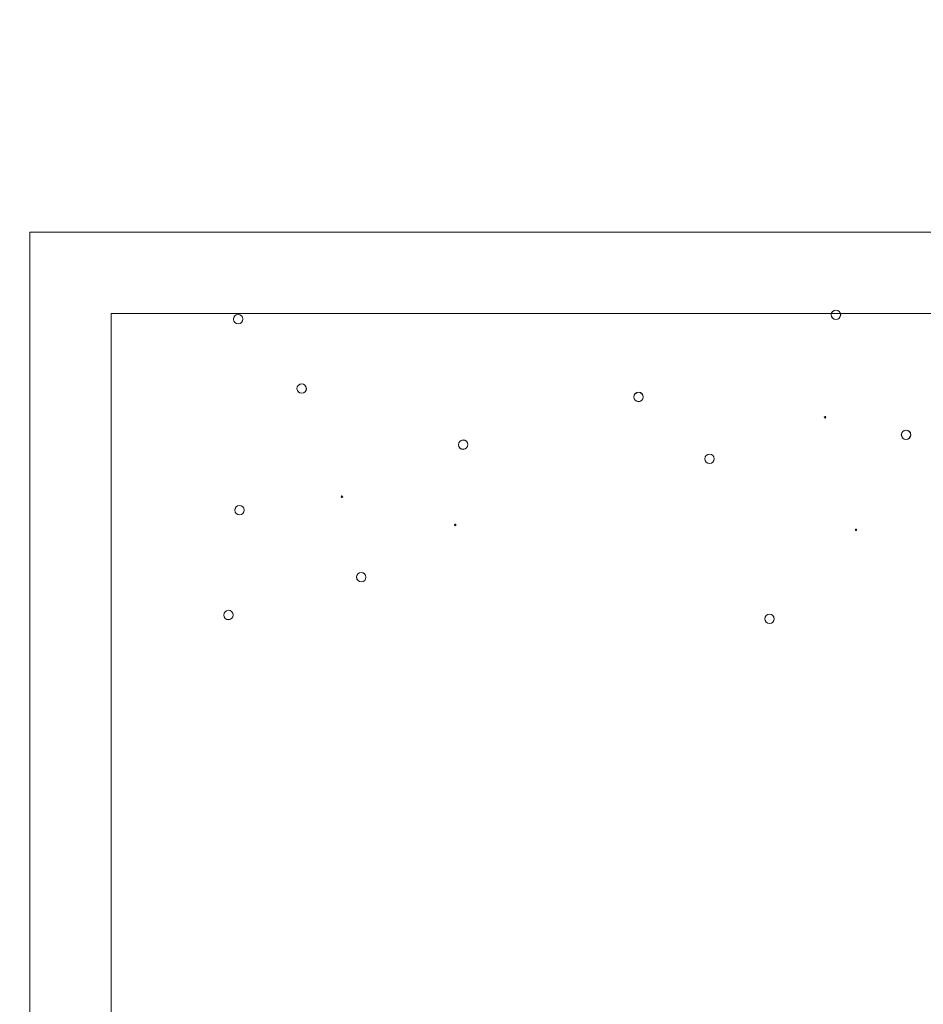
# Model space of a CAD drawing. Units: inches. Extents: x -466983 to 1020, y 324 to 318697.
# Tile 52 of 97: x 620.61 to 631.8, y 936.44 to 948.64. Entities that reach past the tile are written whole.
import ezdxf

# ---------------------------------------------------------------- set-up
doc = ezdxf.new("R2010")
doc.units = ezdxf.units.IN
doc.header["$MEASUREMENT"] = 0
doc.layers.add('A-FLOR-PATT', color=252, linetype='Continuous', lineweight=13)
doc.layers.add('A-FURN', color=8, linetype='Continuous', lineweight=18)

# ---------------------------------------------------------------- blocks, each defined once
blk = doc.blocks.new('L Shaped Sofa')
at = {"ltscale": 2}
for p, q in [((2458.96, 739.532), (2458.96, 802.773)), ((2460.8, 737.692), (2460.8, 802.773)), ((2458.96, 739.532), (2437.956, 739.532)), ((2460.8, 737.692), (2437.499, 737.692))]:
    blk.add_line(p, q, dxfattribs=at)
for centre, radius, start, end in [((2444.081, 746.436), 0.106, 90, 270), ((2444.081, 746.436), 0.106, 270, 90), ((2456.312, 746.349), 0.106, 1.3946, 181.3946), ((2456.312, 746.349), 0.106, 181.3946, 1.3946), ((2453.309, 745.494), 0.106, 1.3946, 181.3946), ((2453.309, 745.494), 0.106, 181.3946, 1.3946), ((2442.129, 744.423), 0.0177, 90, 270), ((2442.129, 744.423), 0.0177, 270, 90), ((2451.187, 744.312), 0.0177, 1.3946, 181.3946), ((2451.187, 744.312), 0.0177, 181.3946, 1.3946), ((2456.062, 743.978), 0.106, 1.3946, 181.3946), ((2456.062, 743.978), 0.106, 181.3946, 1.3946), ((2453.747, 743.675), 0.0177, 1.3946, 181.3946), ((2453.747, 743.675), 0.0177, 181.3946, 1.3946), ((2445.438, 742.815), 0.106, 90, 270), ((2445.438, 742.815), 0.106, 270, 90), ((2451.005, 742.498), 0.106, 1.3946, 181.3946), ((2451.005, 742.498), 0.106, 181.3946, 1.3946), ((2440.998, 742.273), 0.106, 90, 270), ((2440.998, 742.273), 0.106, 270, 90), ((2442.827, 741.879), 0.0177, 90, 270), ((2442.827, 741.879), 0.0177, 270, 90), ((2447.044, 741.419), 0.106, 90, 270), ((2447.044, 741.419), 0.106, 270, 90), ((2454.657, 741.23), 0.106, 1.3946, 181.3946), ((2454.657, 741.23), 0.106, 181.3946, 1.3946), ((2456.093, 739.658), 0.106, 1.3946, 181.3946), ((2442.581, 739.558), 0.106, 90, 270), ((2442.581, 739.558), 0.106, 270, 90), ((2456.093, 739.658), 0.106, 181.3946, 1.3946)]:
    blk.add_arc(centre, radius, start, end, dxfattribs=at)

msp = doc.modelspace()

# ---------------------------------------------------------------- hatches: boundary and pattern name
at = {"layer": 'A-FLOR-PATT', "transparency": 33554572}
h = msp.add_hatch(dxfattribs=at)
h.set_pattern_fill('ANSI37', color=256, scale=30)
h.set_pattern_definition([(45, (-1212.4137, -290.035), (-2.6516504, 2.6516504), []), (135, (-1212.4137, -290.035), (-2.6516504, -2.6516504), [])])
h.paths.add_polyline_path([(901.806, 1075.938), (900.614, 1075.938), (900.614, 1065.386), (899.391, 1065.386), (898.091, 1065.386), (892.836, 1058.71, -0.258377), (892.188, 1058.351), (879.985, 1058.351, -0.20177), (879.438, 1058.581), (874.081, 1065.386), (872.781, 1065.386), (871.558, 1065.386), (871.558, 1075.938), (813.806, 1075.938), (813.806, 1044.792), (832.395, 1044.792, -0.394795), (848.66, 1028.536), (848.66, 1009.938), (901.806, 1009.938), (901.806, 1015.938), (901.306, 1015.938), (871.306, 1015.938), (871.306, 1017.25), (871.334, 1017.25, -0.401453), (901.306, 1045.938), (901.806, 1045.938)])
edge = h.paths.add_edge_path(flags=16)
edge.add_line((847.773, 1068.949), (847.773, 1073.709))
edge.add_arc((849.227, 1073.709), 1.454, 90, 180, ccw=False)
edge.add_line((849.227, 1075.163), (864.492, 1075.163))
edge.add_arc((864.492, 1073.709), 1.454, 0, 90, ccw=False)
edge.add_line((865.946, 1073.709), (865.946, 1069.004))
edge.add_arc((832.645, 1068.976), 33.301, -20.6123, 0.0472, ccw=False)
edge.add_ellipse((856.859, 1058.48), major_axis=(0, 10.213), ratio=0.685919, start_angle=100.0088, end_angle=259.9912, ccw=False)
edge.add_arc((881.074, 1068.976), 33.301, 180.0472, 200.6123, ccw=False)
h.paths.add_polyline_path([(853.146, 1066.482), (853.146, 1066.453), (853.146, 1066.453, 0.433107), (852.917, 1066.685), (852.917, 1066.453), (853.146, 1066.453), (853.146, 1066.482), (853.088, 1066.612, 0.697939), (852.7, 1066.453), (852.7, 1066.453), (852.7, 1066.482), (852.917, 1067.001), (852.917, 1066.685, -0.396254)], flags=0)
h.paths.add_polyline_path([(861.019, 1066.482), (861.019, 1066.453), (861.019, 1066.453, 0.416404), (860.802, 1066.685), (860.802, 1066.453), (861.019, 1066.453), (861.019, 1066.482), (860.967, 1066.605, 0.713344), (860.573, 1066.453), (860.573, 1066.453), (860.573, 1066.482), (860.802, 1067.001), (860.802, 1066.685, -0.379973)], flags=0)
edge = h.paths.add_edge_path(flags=0)
edge.add_spline(control_points=[(861.13, 1065.785), (861.466, 1065.248), (861.613, 1065.016), (861.983, 1064.374), (862.192, 1063.944), (862.561, 1063.039), (862.721, 1062.563), (862.987, 1061.578), (863.092, 1061.069), (863.245, 1060.031), (863.293, 1059.503), (863.329, 1058.441), (863.318, 1057.908), (863.237, 1056.852), (863.166, 1056.329), (862.97, 1055.308), (862.843, 1054.81), (862.537, 1053.852), (862.357, 1053.393), (861.951, 1052.525), (861.725, 1052.117), (861.233, 1051.362), (860.967, 1051.016), (860.405, 1050.395), (860.108, 1050.12), (859.494, 1049.646), (859.176, 1049.448), (858.528, 1049.13), (858.197, 1049.011), (857.531, 1048.852), (857.196, 1048.812), (856.525, 1048.812), (856.189, 1048.852), (855.524, 1049.01), (855.193, 1049.129), (854.545, 1049.447), (854.227, 1049.645), (853.612, 1050.118), (853.316, 1050.393), (852.753, 1051.014), (852.487, 1051.36), (851.995, 1052.114), (851.769, 1052.523), (851.363, 1053.39), (851.183, 1053.85), (850.877, 1054.807), (850.75, 1055.305), (850.553, 1056.326), (850.483, 1056.849), (850.401, 1057.905), (850.39, 1058.438), (850.426, 1059.5), (850.473, 1060.028), (850.626, 1061.066), (850.732, 1061.575), (850.997, 1062.561), (851.157, 1063.036), (851.525, 1063.942), (851.734, 1064.371), (852.106, 1065.016), (852.254, 1065.25), (852.608, 1065.733)], knot_values=[3.915332, 3.915332, 3.915332, 3.915332, 4.013468, 4.013468, 4.175532, 4.175532, 4.337596, 4.337596, 4.49966, 4.49966, 4.661724, 4.661724, 4.823788, 4.823788, 4.985852, 4.985852, 5.147916, 5.147916, 5.30998, 5.30998, 5.472044, 5.472044, 5.634109, 5.634109, 5.796173, 5.796173, 5.958237, 5.958237, 6.120301, 6.120301, 6.282365, 6.282365, 6.444429, 6.444429, 6.606493, 6.606493, 6.768557, 6.768557, 6.930621, 6.930621, 7.092685, 7.092685, 7.254749, 7.254749, 7.416813, 7.416813, 7.578878, 7.578878, 7.740942, 7.740942, 7.903006, 7.903006, 8.06507, 8.06507, 8.227134, 8.227134, 8.389198, 8.389198, 8.551262, 8.551262, 8.65037, 8.65037, 8.65037, 8.65037], degree=3, periodic=0)
edge.add_line((852.642, 1065.785), (861.13, 1065.785))
edge = h.paths.add_edge_path(flags=0)
edge.add_ellipse((856.85, 1057.743), major_axis=(0, 7.792), ratio=0.687861, start_angle=0, end_angle=360)
h.paths.add_polyline_path([(848.863, 1069.389), (848.863, 1073.96, -0.414214), (849.954, 1075.051), (863.765, 1075.051, -0.414214), (864.856, 1073.96), (864.856, 1069.389, -0.388936), (864.524, 1069.027, -0.043561), (849.195, 1069.027, -0.388936)], flags=0)
h.paths.add_polyline_path([(853.101, 1068.112, -1), (852.677, 1068.112, -1)], flags=0)
edge = h.paths.add_edge_path(flags=0)
edge.add_ellipse((856.859, 1057.338), major_axis=(0, 2.207), ratio=0.657164, start_angle=0, end_angle=360)
h.paths.add_polyline_path([(861.041, 1068.112, -1), (860.618, 1068.112, -1)], flags=0)
edge = h.paths.add_edge_path()
edge.add_line((573.954, 1057.341), (573.954, 1075.938))
edge.add_line((573.954, 1075.938), (558.731, 1075.938))
edge.add_line((558.731, 1075.938), (558.731, 1065.386))
edge.add_line((558.731, 1065.386), (557.507, 1065.386))
edge.add_line((557.507, 1065.386), (556.207, 1065.386))
edge.add_line((556.207, 1065.386), (550.952, 1058.71))
edge.add_arc((550.304, 1059.116), 0.765, 270, 327.9483, ccw=False)
edge.add_line((550.304, 1058.351), (538.101, 1058.351))
edge.add_arc((538.101, 1059.116), 0.765, 224.3704, 270, ccw=False)
edge.add_line((537.555, 1058.581), (532.198, 1065.386))
edge.add_line((532.198, 1065.386), (530.898, 1065.386))
edge.add_line((530.898, 1065.386), (529.674, 1065.386))
edge.add_line((529.674, 1065.386), (529.674, 1075.938))
edge.add_line((529.674, 1075.938), (520.806, 1075.938))
edge.add_line((520.806, 1075.938), (520.806, 1045.938))
edge.add_line((520.806, 1045.938), (521.306, 1045.938))
edge.add_arc((521.306, 1015.938), 30, 2.5075, 90, ccw=False)
edge.add_line((551.277, 1017.25), (551.306, 1017.25))
edge.add_line((551.306, 1017.25), (551.306, 1015.938))
edge.add_line((551.306, 1015.938), (520.806, 1015.938))
edge.add_line((520.806, 1015.938), (520.806, 1009.938))
edge.add_line((520.806, 1009.938), (559.191, 1010.402))
edge.add_arc((559.191, 1011.856), 1.454, 180, 270, ccw=False)
edge.add_line((557.737, 1011.856), (557.737, 1016.561))
edge.add_arc((591.039, 1016.589), 33.301, 159.3877, 180.0472, ccw=False)
edge.add_ellipse((566.824, 1027.085), major_axis=(0, 10.213), ratio=0.685919, start_angle=280.0088, end_angle=439.9912, ccw=False)
edge.add_arc((542.609, 1016.589), 33.301, 0.0472, 20.6123, ccw=False)
edge.add_line((575.91, 1016.616), (575.91, 1011.856))
edge.add_arc((574.456, 1011.856), 1.454, -90, 0, ccw=False)
edge.add_line((574.456, 1010.402), (608.806, 1009.938))
edge.add_line((608.806, 1009.938), (608.806, 1041.086))
edge.add_line((608.806, 1041.086), (590.218, 1041.086))
edge.add_arc((590.775, 1057.907), 16.831, 181.9277, 268.1032, ccw=False)
edge = h.paths.add_edge_path()
edge.add_ellipse((494.244, 583.62), major_axis=(0, 10.213), ratio=0.685919, start_angle=280.0088, end_angle=439.9912, ccw=False)
edge.add_arc((470.03, 573.124), 33.301, 0.0472, 20.6123, ccw=False)
edge.add_line((503.331, 573.152), (503.331, 568.392))
edge.add_arc((501.877, 568.392), 1.454, -90, 0, ccw=False)
edge.add_line((501.877, 566.938), (539.806, 566.938))
edge.add_line((539.806, 566.938), (539.806, 572.938))
edge.add_line((539.806, 572.938), (539.306, 572.938))
edge.add_line((539.306, 572.938), (509.306, 572.938))
edge.add_line((509.306, 572.938), (509.306, 574.25))
edge.add_line((509.306, 574.25), (509.334, 574.25))
edge.add_arc((539.306, 572.938), 30, 90, 177.4925, ccw=False)
edge.add_line((539.306, 602.938), (539.806, 602.938))
edge.add_line((539.806, 602.938), (539.806, 626.938))
edge.add_line((539.806, 626.938), (531.772, 626.938))
edge.add_line((531.772, 626.938), (531.772, 616.386))
edge.add_line((531.772, 616.386), (530.548, 616.386))
edge.add_line((530.548, 616.386), (529.249, 616.386))
edge.add_line((529.249, 616.386), (523.711, 609.351))
edge.add_line((523.711, 609.351), (510.777, 609.351))
edge.add_line((510.777, 609.351), (505.239, 616.386))
edge.add_line((505.239, 616.386), (503.939, 616.386))
edge.add_line((503.939, 616.386), (502.715, 616.386))
edge.add_line((502.715, 616.386), (502.715, 626.938))
edge.add_line((502.715, 626.938), (481.698, 626.938))
edge.add_line((481.698, 626.938), (481.698, 610.995))
edge.add_arc((467.27, 611.473), 14.436, 271.9277, 358.1032, ccw=False)
edge.add_line((467.756, 597.045), (451.806, 597.045))
edge.add_line((451.806, 597.045), (451.806, 584.404))
edge.add_line((451.806, 584.404), (451.806, 566.938))
edge.add_line((451.806, 566.938), (486.612, 566.938))
edge.add_arc((486.612, 568.392), 1.454, 180, 270, ccw=False)
edge.add_line((485.158, 568.392), (485.158, 573.097))
edge.add_arc((518.459, 573.124), 33.301, 159.3877, 180.0472, ccw=False)
h.paths.add_polyline_path([(836.261, 1020.733), (879.89, 1020.733), (879.89, 1039.39), (836.261, 1039.39)], flags=25)
h.paths.add_polyline_path([(549.985, 1036.749), (593.614, 1036.749), (593.614, 1055.407), (549.985, 1055.407)], flags=24)
h.paths.add_polyline_path([(475.123, 595.596), (518.752, 595.596), (518.752, 614.253), (475.123, 614.253)], flags=24)
h = msp.add_hatch(dxfattribs=at)
h.set_pattern_fill('ANSI37', color=256, scale=20)
h.set_pattern_definition([(45, (-1212.4137, -290.035), (-1.767767, 1.767767), []), (135, (-1212.4137, -290.035), (-1.767767, -1.767767), [])])
h.paths.add_polyline_path([(809.806, 870.938), (809.806, 888.152), (806.998, 888.152), (802.662, 888.152), (789.383, 888.152), (786.285, 888.152, -0.414214), (785.499, 888.937), (785.499, 900.196), (785.499, 908.47, -0.414214), (786.808, 909.779, -0.414214), (785.499, 911.088), (785.499, 929.101, -0.414214), (786.808, 930.411, -0.414214), (785.499, 931.72), (785.499, 931.904, -0.414214), (784.19, 930.595), (766.722, 930.595, -0.412359), (765.413, 931.896, -0.413741), (764.115, 930.578), (744.578, 930.422, -0.416556), (743.786, 931.207), (743.786, 933.515), (742.215, 933.515), (742.215, 952.024, -0.001344), (743.786, 952.2), (743.786, 953.938), (678.592, 953.938), (678.592, 951.131), (678.592, 946.794), (678.592, 933.515), (678.592, 930.417, -0.414214), (677.806, 929.631), (666.548, 929.631), (658.274, 929.631, -0.414214), (656.965, 930.94, -0.414214), (655.656, 929.631), (637.642, 929.631, -0.414214), (636.333, 930.94, -0.414214), (635.024, 929.631), (634.839, 929.631, -0.414214), (636.149, 928.322), (636.149, 910.854, -0.412359), (634.848, 909.545, -0.413741), (636.165, 908.247), (636.321, 888.71, -0.416556), (635.536, 887.918), (633.228, 887.918), (633.228, 886.347), (614.719, 886.347, -0.001344), (614.544, 887.918), (612.806, 887.918), (612.806, 834.938), (612.806, 752.938), (612.806, 748.938), (612.806, 697.938), (654.806, 697.938), (654.806, 701.938), (715.806, 701.938), (715.806, 737.435), (774.292, 737.435), (774.292, 795.938), (809.806, 795.938)])
h.paths.add_polyline_path([(679.276, 849.576, 0.102523), (682.148, 849.261, -0.080461), (694.543, 849.773, -0.283899), (694.482, 849.008, 0.136605), (694.407, 848.81, -0.030441), (694.543, 846.893), (694.543, 842.62), (694.543, 838.347, -0.028219), (694.425, 836.568), (694.425, 836.568, 0.196187), (694.446, 836.271, -0.302897), (694.543, 835.467, -0.080461), (682.148, 835.979, 0.102523), (679.276, 835.664, -0.58611), (678.646, 836.017), (678.646, 849.223, -0.58611)], flags=16)
h.paths.add_polyline_path([(679.517, 848.651, 0.699597), (679.476, 848.634, 1.20716), (679.194, 848.742, 0.010621)], flags=0)
h.paths.add_polyline_path([(679.492, 836.561, -0.013798), (679.918, 836.659, -0.071703), (682.853, 837.143, -0.165743), (682.166, 839.101), (682.166, 842.609), (682.166, 846.06, -0.240616), (683.473, 848.677, -0.068263), (693.929, 849.008), (693.788, 848.708), (693.788, 849.023, 0.067332), (683.473, 848.677, 0.240616), (682.166, 846.06), (682.166, 842.609), (682.166, 839.101, 0.23459), (683.461, 836.551, 0.068093), (693.788, 836.195), (693.788, 836.51), (693.93, 836.21, -0.077215), (682.242, 836.782, 0.086627), (679.528, 836.57, -0.628402), (679.503, 836.573), (679.503, 836.607, 0.910458)], flags=0)
h.paths.add_polyline_path([(679.476, 848.636), (679.207, 848.647), (679.207, 836.572, 0.913566), (679.365, 836.586), (679.476, 836.582)], flags=0)
h.paths.add_polyline_path([(679.276, 829.86, 0.102523), (682.148, 829.546, -0.080461), (694.543, 830.057, -0.283899), (694.482, 829.293, 0.136605), (694.407, 829.095, -0.030441), (694.543, 827.178), (694.543, 822.904), (694.543, 818.631, -0.028219), (694.425, 816.853), (694.425, 816.853, 0.196187), (694.446, 816.556, -0.302897), (694.543, 815.752, -0.080461), (682.148, 816.263, 0.102523), (679.276, 815.949, -0.58611), (678.646, 816.302), (678.646, 829.507, -0.58611)], flags=16)
h.paths.add_polyline_path([(679.517, 828.936, 0.699597), (679.476, 828.919, 1.20716), (679.194, 829.027, 0.010621)], flags=0)
h.paths.add_polyline_path([(679.492, 816.846, -0.013798), (679.918, 816.944, -0.071703), (682.853, 817.428, -0.165743), (682.166, 819.385), (682.166, 822.894), (682.166, 826.345, -0.240616), (683.473, 828.961, -0.068263), (693.929, 829.293), (693.788, 828.993), (693.788, 829.308, 0.067332), (683.473, 828.961, 0.240616), (682.166, 826.345), (682.166, 822.894), (682.166, 819.385, 0.23459), (683.461, 816.836, 0.068093), (693.788, 816.48), (693.788, 816.795), (693.93, 816.495, -0.077215), (682.242, 817.066, 0.086627), (679.528, 816.855, -0.628402), (679.503, 816.858), (679.503, 816.892, 0.910458)], flags=0)
h.paths.add_polyline_path([(679.476, 828.921), (679.207, 828.932), (679.207, 816.857, 0.913566), (679.365, 816.871), (679.476, 816.867)], flags=0)
h.paths.add_polyline_path([(679.276, 810.145, 0.102523), (682.148, 809.83, -0.080461), (694.543, 810.342, -0.3023), (694.447, 809.539, 0.10023), (694.406, 809.388, -0.03057), (694.543, 807.462), (694.543, 803.189), (694.543, 798.916, -0.03057), (694.406, 796.991, 0.10023), (694.447, 796.839, -0.3023), (694.543, 796.036, -0.080461), (682.148, 796.548, 0.102523), (679.276, 796.233, -0.58611), (678.646, 796.586), (678.646, 809.792, -0.58611)], flags=16)
h.paths.add_polyline_path([(679.517, 809.242, 0.699597), (679.476, 809.224, 1.20716), (679.194, 809.332, 0.010621)], flags=0)
h.paths.add_polyline_path([(679.492, 797.151, -0.013798), (679.918, 797.25, -0.071703), (682.853, 797.734, -0.165743), (682.166, 799.691), (682.166, 803.2), (682.166, 806.65, -0.239349), (683.461, 809.258, -0.072465), (694.447, 809.541, 0.197932), (694.425, 809.241), (693.788, 809.299), (693.788, 809.614, 0.068093), (683.461, 809.258, 0.239349), (682.166, 806.65), (682.166, 803.2), (682.166, 799.691, 0.235854), (683.473, 797.132, 0.067332), (693.788, 796.786), (693.788, 797.101), (694.425, 797.159, 0.197932), (694.447, 796.859, -0.080419), (682.156, 797.379, 0.083867), (679.528, 797.16, -0.628402), (679.503, 797.164), (679.503, 797.197, 0.910458)], flags=0)
h.paths.add_polyline_path([(679.207, 809.237), (679.207, 797.162, 0.913566), (679.365, 797.176), (679.476, 797.173), (679.476, 809.227)], flags=0)
h.paths.add_polyline_path([(695.364, 853.299), (728.223, 853.299), (728.223, 771.152), (695.364, 771.152)], flags=16)
h.paths.add_polyline_path([(696.021, 852.642), (727.566, 852.642), (727.566, 771.809), (696.021, 771.809)], flags=0)
h.paths.add_polyline_path([(679.276, 788.787, 0.102523), (682.148, 788.472, -0.080461), (694.543, 788.984, -0.3023), (694.447, 788.181, 0.10023), (694.406, 788.03, -0.03057), (694.543, 786.104), (694.543, 781.831), (694.543, 777.558, -0.03057), (694.406, 775.632, 0.10023), (694.447, 775.481, -0.3023), (694.543, 774.678, -0.080461), (682.148, 775.19, 0.102523), (679.276, 774.875, -0.58611), (678.646, 775.228), (678.646, 788.434, -0.58611)], flags=16)
h.paths.add_polyline_path([(679.517, 787.883, 0.699597), (679.476, 787.866, 1.20716), (679.194, 787.974, 0.010621)], flags=0)
h.paths.add_polyline_path([(679.492, 775.793, -0.013798), (679.918, 775.891, -0.071703), (682.853, 776.375, -0.165743), (682.166, 778.333), (682.166, 781.841), (682.166, 785.292, -0.239349), (683.461, 787.899, -0.072465), (694.447, 788.182, 0.197932), (694.425, 787.882), (693.788, 787.94), (693.788, 788.255, 0.068093), (683.461, 787.899, 0.239349), (682.166, 785.292), (682.166, 781.841), (682.166, 778.333, 0.235854), (683.473, 775.774, 0.067332), (693.788, 775.428), (693.788, 775.742), (694.425, 775.8, 0.197932), (694.447, 775.5, -0.080419), (682.156, 776.021, 0.083867), (679.528, 775.802, -0.628402), (679.503, 775.805), (679.503, 775.839, 0.910458)], flags=0)
h.paths.add_polyline_path([(679.207, 787.879), (679.207, 775.804, 0.913566), (679.365, 775.818), (679.476, 775.814), (679.476, 787.868)], flags=0)
h.paths.add_polyline_path([(704.641, 854.12, -0.080461), (705.153, 866.516, 0.102523), (704.838, 869.387, -0.58611), (705.191, 870.017), (718.397, 870.017, -0.58611), (718.75, 869.387, 0.102523), (718.435, 866.516, -0.080461), (718.946, 854.12, -0.3023), (718.144, 854.217, 0.10023), (717.992, 854.257, -0.03057), (716.067, 854.12), (711.794, 854.12), (707.521, 854.12, -0.03057), (705.595, 854.257, 0.10023), (705.444, 854.217, -0.3023)], flags=16)
h.paths.add_polyline_path([(717.846, 869.146, 0.699597), (717.829, 869.187, 1.20716), (717.937, 869.47, 0.010621)], flags=0)
h.paths.add_polyline_path([(705.463, 854.216, -0.080419), (705.984, 866.507, 0.083867), (705.765, 869.135, -0.628402), (705.768, 869.16), (705.802, 869.16, 0.910458), (705.756, 869.171, -0.013798), (705.854, 868.745, -0.071703), (706.338, 865.81, -0.165743), (708.295, 866.497), (711.804, 866.497), (715.255, 866.497, -0.239349), (717.862, 865.202, -0.072465), (718.145, 854.216, 0.197932), (717.845, 854.238), (717.903, 854.876), (718.218, 854.876, 0.068093), (717.862, 865.202, 0.239349), (715.255, 866.497), (711.804, 866.497), (708.295, 866.497, 0.235854), (705.737, 865.19, 0.067332), (705.391, 854.876), (705.705, 854.876), (705.763, 854.238, 0.197932)], flags=16)
h.paths.add_polyline_path([(705.766, 869.456, 0.913566), (705.781, 869.299), (705.777, 869.187), (717.831, 869.187), (717.842, 869.456)], flags=0)
h.paths.add_polyline_path([(729.045, 842.62), (729.045, 846.893, -0.03057), (729.182, 848.818, 0.10023), (729.141, 848.97, -0.3023), (729.045, 849.773, -0.080461), (741.44, 849.261, 0.102523), (744.311, 849.576, -0.58611), (744.942, 849.223), (744.942, 836.017, -0.58611), (744.311, 835.664, 0.102523), (741.44, 835.979, -0.080461), (729.045, 835.467, -0.3023), (729.141, 836.27, 0.10023), (729.182, 836.421, -0.03057), (729.045, 838.347)], flags=16)
h.paths.add_polyline_path([(744.111, 836.585, 1.20716), (744.394, 836.477, 0.010621), (744.07, 836.567, 0.699597)], flags=0)
h.paths.add_polyline_path([(729.141, 836.268, 0.197932), (729.162, 836.568), (729.8, 836.51), (729.8, 836.195, 0.068093), (740.126, 836.551, 0.239349), (741.421, 839.159), (741.421, 842.609), (741.421, 846.118, 0.235854), (740.114, 848.677, 0.067332), (729.8, 849.023), (729.8, 848.708), (729.162, 848.65, 0.197932), (729.141, 848.95, -0.080419), (741.432, 848.43, 0.083867), (744.059, 848.649, -0.628402), (744.085, 848.645), (744.085, 848.612, 0.910458), (744.095, 848.658, -0.013798), (743.67, 848.559, -0.071703), (740.734, 848.075, -0.165743), (741.421, 846.118), (741.421, 842.609), (741.421, 839.159, -0.239349), (740.126, 836.551, -0.072465)], flags=0)
h.paths.add_polyline_path([(729.045, 830.057, -0.080461), (741.44, 829.546, 0.102523), (744.311, 829.86, -0.58611), (744.942, 829.507), (744.942, 816.302, -0.58611), (744.311, 815.949, 0.102523), (741.44, 816.263, -0.080461), (729.045, 815.752, -0.3023), (729.141, 816.554, 0.10023), (729.182, 816.706, -0.03057), (729.045, 818.631), (729.045, 822.904), (729.045, 827.178, -0.03057), (729.182, 829.103, 0.10023), (729.141, 829.255, -0.3023)], flags=16)
h.paths.add_polyline_path([(744.111, 816.869, 1.20716), (744.394, 816.761, 0.010621), (744.07, 816.852, 0.699597)], flags=0)
h.paths.add_polyline_path([(729.141, 829.235, -0.080419), (741.432, 828.714, 0.083867), (744.059, 828.933, -0.628402), (744.085, 828.93), (744.085, 828.896, 0.910458), (744.095, 828.943, -0.013798), (743.67, 828.844, -0.071703), (740.734, 828.36, -0.165743), (741.421, 826.403), (741.421, 822.894), (741.421, 819.443, -0.239349), (740.126, 816.836, -0.072465), (729.141, 816.553, 0.197932), (729.162, 816.853), (729.8, 816.795), (729.8, 816.48, 0.068093), (740.126, 816.836, 0.239349), (741.421, 819.443), (741.421, 822.894), (741.421, 826.403, 0.235854), (740.114, 828.961, 0.067332), (729.8, 829.308), (729.8, 828.993), (729.162, 828.935, 0.197932)], flags=16)
h.paths.add_polyline_path([(729.045, 810.342, -0.080461), (741.44, 809.83, 0.102523), (744.311, 810.145, -0.58611), (744.942, 809.792), (744.942, 796.586, -0.58611), (744.311, 796.233, 0.102523), (741.44, 796.548, -0.080461), (729.045, 796.036, -0.283899), (729.105, 796.801, 0.136605), (729.181, 796.999, -0.030441), (729.045, 798.916), (729.045, 803.189), (729.045, 807.462, -0.028219), (729.163, 809.241), (729.162, 809.241, 0.196187), (729.142, 809.538, -0.302897)], flags=16)
h.paths.add_polyline_path([(744.111, 797.175, 1.20716), (744.394, 797.067, 0.010621), (744.07, 797.158, 0.699597)], flags=0)
h.paths.add_polyline_path([(741.345, 809.027, 0.086627), (744.059, 809.239, -0.628402), (744.085, 809.235), (744.085, 809.202, 0.910458), (744.095, 809.248, -0.013798), (743.67, 809.15, -0.071703), (740.734, 808.666, -0.165743), (741.421, 806.708), (741.421, 803.2), (741.421, 799.749, -0.240616), (740.114, 797.132, -0.068263), (729.658, 796.801), (729.8, 797.101), (729.8, 796.786, 0.067332), (740.114, 797.132, 0.240616), (741.421, 799.749), (741.421, 803.2), (741.421, 806.708, 0.23459), (740.126, 809.258, 0.068093), (729.8, 809.614), (729.8, 809.299), (729.658, 809.599, -0.077215)], flags=0)
h.paths.add_polyline_path([(704.641, 770.33, -0.283899), (705.405, 770.27, 0.136605), (705.603, 770.194, -0.030441), (707.521, 770.33), (711.794, 770.33), (716.067, 770.33, -0.028219), (717.845, 770.212), (717.845, 770.213, 0.196187), (718.143, 770.233, -0.302897), (718.946, 770.33, -0.080461), (718.435, 757.935, 0.102523), (718.75, 755.064, -0.58611), (718.397, 754.433), (705.191, 754.433, -0.58611), (704.838, 755.064, 0.102523), (705.153, 757.935, -0.080461)], flags=16)
h.paths.add_polyline_path([(705.762, 755.305, 0.699597), (705.779, 755.264, 1.20716), (705.671, 754.981, 0.010621)], flags=0)
h.paths.add_polyline_path([(705.405, 769.717), (705.705, 769.575), (705.391, 769.575, 0.067332), (705.737, 759.261, 0.240616), (708.353, 757.954), (711.804, 757.954), (715.313, 757.954, 0.23459), (717.862, 759.249, 0.068093), (718.218, 769.575), (717.903, 769.575), (718.203, 769.717, -0.077215), (717.632, 758.03, 0.086627), (717.843, 755.316, -0.628402), (717.84, 755.29), (717.806, 755.29, 0.910458), (717.853, 755.28, -0.013798), (717.754, 755.705, -0.071703), (717.27, 758.641, -0.165743), (715.313, 757.954), (711.804, 757.954), (708.353, 757.954, -0.240616), (705.737, 759.261, -0.068263)], flags=0)
h.paths.add_polyline_path([(729.045, 788.984, -0.080461), (741.44, 788.472, 0.102523), (744.311, 788.787, -0.58611), (744.942, 788.434), (744.942, 775.228, -0.58611), (744.311, 774.875, 0.102523), (741.44, 775.19, -0.080461), (729.045, 774.678, -0.283899), (729.105, 775.443, 0.136605), (729.181, 775.64, -0.030441), (729.045, 777.558), (729.045, 781.831), (729.045, 786.104, -0.028219), (729.163, 787.882), (729.162, 787.882, 0.196187), (729.142, 788.18, -0.302897)], flags=16)
h.paths.add_polyline_path([(744.111, 775.817, 1.20716), (744.394, 775.709, 0.010621), (744.07, 775.799, 0.699597)], flags=0)
h.paths.add_polyline_path([(741.345, 787.669, 0.086627), (744.059, 787.881, -0.628402), (744.085, 787.877), (744.085, 787.844, 0.910458), (744.095, 787.89, -0.013798), (743.67, 787.791, -0.071703), (740.734, 787.307, -0.165743), (741.421, 785.35), (741.421, 781.841), (741.421, 778.39, -0.240616), (740.114, 775.774, -0.068263), (729.658, 775.443), (729.8, 775.742), (729.8, 775.428, 0.067332), (740.114, 775.774, 0.240616), (741.421, 778.39), (741.421, 781.841), (741.421, 785.35, 0.23459), (740.126, 787.899, 0.068093), (729.8, 788.255), (729.8, 787.94), (729.658, 788.241, -0.077215)], flags=0)
h.paths.add_polyline_path([(744.111, 848.636), (744.111, 836.582), (744.381, 836.572), (744.381, 848.647, 0.913566), (744.223, 848.633)], flags=0)
h.paths.add_polyline_path([(744.223, 828.917), (744.111, 828.921), (744.111, 816.867), (744.381, 816.857), (744.381, 828.932, 0.913566)], flags=0)
h.paths.add_polyline_path([(717.831, 755.264), (705.777, 755.264), (705.766, 754.994), (717.842, 754.994, 0.913566), (717.827, 755.152)], flags=0)
h.paths.add_polyline_path([(744.223, 809.223), (744.111, 809.227), (744.111, 797.173), (744.381, 797.162), (744.381, 809.237, 0.913566)], flags=0)
h.paths.add_polyline_path([(744.111, 787.868), (744.111, 775.814), (744.381, 775.804), (744.381, 787.879, 0.913566), (744.223, 787.865)], flags=0)
h.paths.add_polyline_path([(678.877, 877.123), (737.613, 877.123), (737.613, 899.512), (678.877, 899.512)], flags=24)

# ---------------------------------------------------------------- linework, layer by layer
at = {"layer": 'A-FURN', "ltscale": 2}
for p, q in [((620.734, 946.009), (620.734, 910.331)), ((620.734, 946.009), (633.508, 946.009)), ((620.734, 946.009), (620.734, 910.331)), ((620.734, 946.009), (633.508, 946.009)), ((620.734, 946.009), (620.734, 910.331)), ((620.734, 946.009), (633.508, 946.009)), ((620.734, 946.009), (620.734, 910.331)), ((620.734, 946.009), (633.508, 946.009)), ((620.734, 946.009), (620.734, 910.331)), ((620.734, 946.009), (633.508, 946.009)), ((620.734, 946.009), (620.734, 910.331)), ((620.734, 946.009), (633.508, 946.009)), ((621.743, 945), (621.743, 910.331)), ((621.743, 945), (633.258, 945)), ((621.743, 945), (621.743, 910.331)), ((621.743, 945), (633.258, 945)), ((621.743, 945), (621.743, 910.331)), ((621.743, 945), (633.258, 945)), ((621.743, 945), (621.743, 910.331)), ((621.743, 945), (633.258, 945)), ((621.743, 945), (621.743, 910.331)), ((621.743, 945), (633.258, 945)), ((621.743, 945), (621.743, 910.331)), ((621.743, 945), (633.258, 945))]:
    msp.add_line(p, q, dxfattribs=at)
for centre, radius, start, end in [((623.315, 944.931), 0.0582, 1.3946, 181.3946), ((623.315, 944.931), 0.0582, 1.3946, 181.3946), ((623.315, 944.931), 0.0582, 1.3946, 181.3946), ((623.315, 944.931), 0.0582, 1.3946, 181.3946), ((623.315, 944.931), 0.0582, 1.3946, 181.3946), ((623.315, 944.931), 0.0582, 1.3946, 181.3946), ((630.722, 944.986), 0.0582, 90, 270), ((630.722, 944.986), 0.0582, 90, 270), ((630.722, 944.986), 0.0582, 90, 270), ((630.722, 944.986), 0.0582, 90, 270), ((630.722, 944.986), 0.0582, 90, 270), ((630.722, 944.986), 0.0582, 90, 270), ((630.722, 944.986), 0.0582, 270, 90), ((630.722, 944.986), 0.0582, 270, 90), ((630.722, 944.986), 0.0582, 270, 90), ((630.722, 944.986), 0.0582, 270, 90), ((630.722, 944.986), 0.0582, 270, 90), ((630.722, 944.986), 0.0582, 270, 90), ((623.315, 944.931), 0.0582, 181.3946, 1.3946), ((623.315, 944.931), 0.0582, 181.3946, 1.3946), ((623.315, 944.931), 0.0582, 181.3946, 1.3946), ((623.315, 944.931), 0.0582, 181.3946, 1.3946), ((623.315, 944.931), 0.0582, 181.3946, 1.3946), ((623.315, 944.931), 0.0582, 181.3946, 1.3946), ((624.102, 944.07), 0.0582, 1.3946, 181.3946), ((624.102, 944.07), 0.0582, 1.3946, 181.3946), ((624.102, 944.07), 0.0582, 1.3946, 181.3946), ((624.102, 944.07), 0.0582, 1.3946, 181.3946), ((624.102, 944.07), 0.0582, 1.3946, 181.3946), ((624.102, 944.07), 0.0582, 1.3946, 181.3946), ((624.102, 944.07), 0.0582, 181.3946, 1.3946), ((624.102, 944.07), 0.0582, 181.3946, 1.3946), ((624.102, 944.07), 0.0582, 181.3946, 1.3946), ((624.102, 944.07), 0.0582, 181.3946, 1.3946), ((624.102, 944.07), 0.0582, 181.3946, 1.3946), ((624.102, 944.07), 0.0582, 181.3946, 1.3946), ((628.276, 943.966), 0.0582, 90, 270), ((628.276, 943.966), 0.0582, 90, 270), ((628.276, 943.966), 0.0582, 90, 270), ((628.276, 943.966), 0.0582, 90, 270), ((628.276, 943.966), 0.0582, 90, 270), ((628.276, 943.966), 0.0582, 90, 270), ((628.276, 943.966), 0.0582, 270, 90), ((628.276, 943.966), 0.0582, 270, 90), ((628.276, 943.966), 0.0582, 270, 90), ((628.276, 943.966), 0.0582, 270, 90), ((628.276, 943.966), 0.0582, 270, 90), ((628.276, 943.966), 0.0582, 270, 90), ((630.587, 943.714), 0.0097, 90, 270), ((630.587, 943.714), 0.0097, 90, 270), ((630.587, 943.714), 0.0097, 90, 270), ((630.587, 943.714), 0.0097, 90, 270), ((630.587, 943.714), 0.0097, 90, 270), ((630.587, 943.714), 0.0097, 90, 270), ((630.587, 943.714), 0.0097, 270, 90), ((630.587, 943.714), 0.0097, 270, 90), ((630.587, 943.714), 0.0097, 270, 90), ((630.587, 943.714), 0.0097, 270, 90), ((630.587, 943.714), 0.0097, 270, 90), ((630.587, 943.714), 0.0097, 270, 90), ((631.59, 943.498), 0.0582, 90, 270), ((631.59, 943.498), 0.0582, 90, 270), ((631.59, 943.498), 0.0582, 90, 270), ((631.59, 943.498), 0.0582, 90, 270), ((631.59, 943.498), 0.0582, 90, 270), ((631.59, 943.498), 0.0582, 90, 270), ((631.59, 943.498), 0.0582, 270, 90), ((631.59, 943.498), 0.0582, 270, 90), ((631.59, 943.498), 0.0582, 270, 90), ((631.59, 943.498), 0.0582, 270, 90), ((631.59, 943.498), 0.0582, 270, 90), ((631.59, 943.498), 0.0582, 270, 90), ((626.104, 943.375), 0.0582, 1.3946, 181.3946), ((626.104, 943.375), 0.0582, 1.3946, 181.3946), ((626.104, 943.375), 0.0582, 1.3946, 181.3946), ((626.104, 943.375), 0.0582, 1.3946, 181.3946), ((626.104, 943.375), 0.0582, 1.3946, 181.3946), ((626.104, 943.375), 0.0582, 1.3946, 181.3946), ((626.104, 943.375), 0.0582, 181.3946, 1.3946), ((626.104, 943.375), 0.0582, 181.3946, 1.3946), ((626.104, 943.375), 0.0582, 181.3946, 1.3946), ((626.104, 943.375), 0.0582, 181.3946, 1.3946), ((626.104, 943.375), 0.0582, 181.3946, 1.3946), ((626.104, 943.375), 0.0582, 181.3946, 1.3946), ((629.156, 943.2), 0.0582, 90, 270), ((629.156, 943.2), 0.0582, 90, 270), ((629.156, 943.2), 0.0582, 90, 270), ((629.156, 943.2), 0.0582, 90, 270), ((629.156, 943.2), 0.0582, 90, 270), ((629.156, 943.2), 0.0582, 90, 270), ((629.156, 943.2), 0.0582, 270, 90), ((629.156, 943.2), 0.0582, 270, 90), ((629.156, 943.2), 0.0582, 270, 90), ((629.156, 943.2), 0.0582, 270, 90), ((629.156, 943.2), 0.0582, 270, 90), ((629.156, 943.2), 0.0582, 270, 90), ((624.601, 942.729), 0.0097, 1.3946, 181.3946), ((624.601, 942.729), 0.0097, 1.3946, 181.3946), ((624.601, 942.729), 0.0097, 1.3946, 181.3946), ((624.601, 942.729), 0.0097, 1.3946, 181.3946), ((624.601, 942.729), 0.0097, 1.3946, 181.3946), ((624.601, 942.729), 0.0097, 1.3946, 181.3946), ((624.601, 942.729), 0.0097, 181.3946, 1.3946), ((624.601, 942.729), 0.0097, 181.3946, 1.3946), ((624.601, 942.729), 0.0097, 181.3946, 1.3946), ((624.601, 942.729), 0.0097, 181.3946, 1.3946), ((624.601, 942.729), 0.0097, 181.3946, 1.3946), ((624.601, 942.729), 0.0097, 181.3946, 1.3946), ((623.332, 942.563), 0.0582, 1.3946, 181.3946), ((623.332, 942.563), 0.0582, 1.3946, 181.3946), ((623.332, 942.563), 0.0582, 1.3946, 181.3946), ((623.332, 942.563), 0.0582, 1.3946, 181.3946), ((623.332, 942.563), 0.0582, 1.3946, 181.3946), ((623.332, 942.563), 0.0582, 1.3946, 181.3946), ((623.332, 942.563), 0.0582, 181.3946, 1.3946), ((623.332, 942.563), 0.0582, 181.3946, 1.3946), ((623.332, 942.563), 0.0582, 181.3946, 1.3946), ((623.332, 942.563), 0.0582, 181.3946, 1.3946), ((623.332, 942.563), 0.0582, 181.3946, 1.3946), ((623.332, 942.563), 0.0582, 181.3946, 1.3946), ((626.004, 942.38), 0.0097, 1.3946, 181.3946), ((626.004, 942.38), 0.0097, 1.3946, 181.3946), ((626.004, 942.38), 0.0097, 1.3946, 181.3946), ((626.004, 942.38), 0.0097, 1.3946, 181.3946), ((626.004, 942.38), 0.0097, 1.3946, 181.3946), ((626.004, 942.38), 0.0097, 1.3946, 181.3946), ((626.004, 942.38), 0.0097, 181.3946, 1.3946), ((626.004, 942.38), 0.0097, 181.3946, 1.3946), ((626.004, 942.38), 0.0097, 181.3946, 1.3946), ((626.004, 942.38), 0.0097, 181.3946, 1.3946), ((626.004, 942.38), 0.0097, 181.3946, 1.3946), ((626.004, 942.38), 0.0097, 181.3946, 1.3946), ((630.97, 942.319), 0.0097, 90, 270), ((630.97, 942.319), 0.0097, 90, 270), ((630.97, 942.319), 0.0097, 90, 270), ((630.97, 942.319), 0.0097, 90, 270), ((630.97, 942.319), 0.0097, 90, 270), ((630.97, 942.319), 0.0097, 90, 270), ((630.97, 942.319), 0.0097, 270, 90), ((630.97, 942.319), 0.0097, 270, 90), ((630.97, 942.319), 0.0097, 270, 90), ((630.97, 942.319), 0.0097, 270, 90), ((630.97, 942.319), 0.0097, 270, 90), ((630.97, 942.319), 0.0097, 270, 90), ((624.841, 941.732), 0.0582, 1.3946, 181.3946), ((624.841, 941.732), 0.0582, 1.3946, 181.3946), ((624.841, 941.732), 0.0582, 1.3946, 181.3946), ((624.841, 941.732), 0.0582, 1.3946, 181.3946), ((624.841, 941.732), 0.0582, 1.3946, 181.3946), ((624.841, 941.732), 0.0582, 1.3946, 181.3946), ((624.841, 941.732), 0.0582, 181.3946, 1.3946), ((624.841, 941.732), 0.0582, 181.3946, 1.3946), ((624.841, 941.732), 0.0582, 181.3946, 1.3946), ((624.841, 941.732), 0.0582, 181.3946, 1.3946), ((624.841, 941.732), 0.0582, 181.3946, 1.3946), ((624.841, 941.732), 0.0582, 181.3946, 1.3946), ((623.195, 941.263), 0.0582, 1.3946, 181.3946), ((623.195, 941.263), 0.0582, 1.3946, 181.3946), ((623.195, 941.263), 0.0582, 1.3946, 181.3946), ((623.195, 941.263), 0.0582, 1.3946, 181.3946), ((623.195, 941.263), 0.0582, 1.3946, 181.3946), ((623.195, 941.263), 0.0582, 1.3946, 181.3946), ((623.195, 941.263), 0.0582, 181.3946, 1.3946), ((623.195, 941.263), 0.0582, 181.3946, 1.3946), ((623.195, 941.263), 0.0582, 181.3946, 1.3946), ((623.195, 941.263), 0.0582, 181.3946, 1.3946), ((623.195, 941.263), 0.0582, 181.3946, 1.3946), ((623.195, 941.263), 0.0582, 181.3946, 1.3946), ((629.9, 941.216), 0.0582, 90, 270), ((629.9, 941.216), 0.0582, 90, 270), ((629.9, 941.216), 0.0582, 90, 270), ((629.9, 941.216), 0.0582, 90, 270), ((629.9, 941.216), 0.0582, 90, 270), ((629.9, 941.216), 0.0582, 90, 270), ((629.9, 941.216), 0.0582, 270, 90), ((629.9, 941.216), 0.0582, 270, 90), ((629.9, 941.216), 0.0582, 270, 90), ((629.9, 941.216), 0.0582, 270, 90), ((629.9, 941.216), 0.0582, 270, 90), ((629.9, 941.216), 0.0582, 270, 90)]:
    msp.add_arc(centre, radius, start, end, dxfattribs=at)

# ---------------------------------------------------------------- block references
at = {"layer": 'A-FURN', "xscale": 0.5482153745360612, "yscale": 0.5482153745360612, "zscale": 0.5482153745360612, "rotation": 180}
msp.add_blockref('L Shaped Sofa', (1969.783, 1350.423), dxfattribs=at)

doc.saveas('drawing.dxf')
